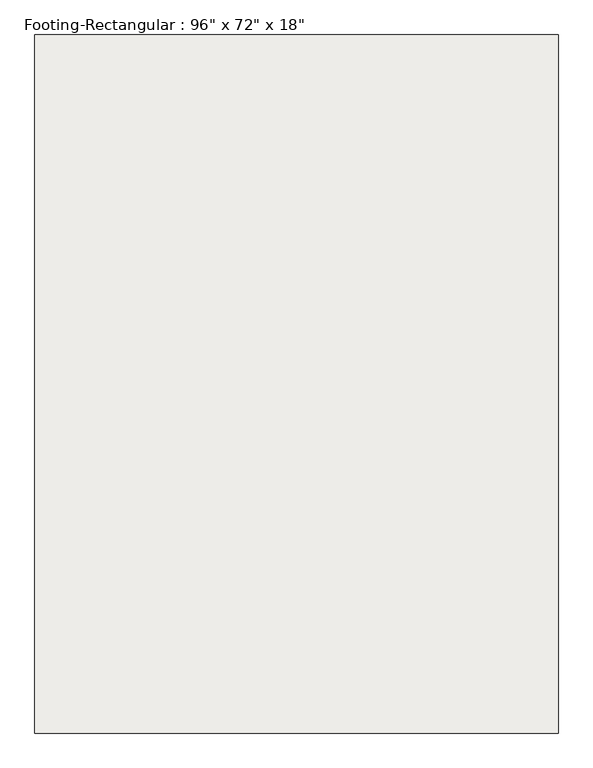
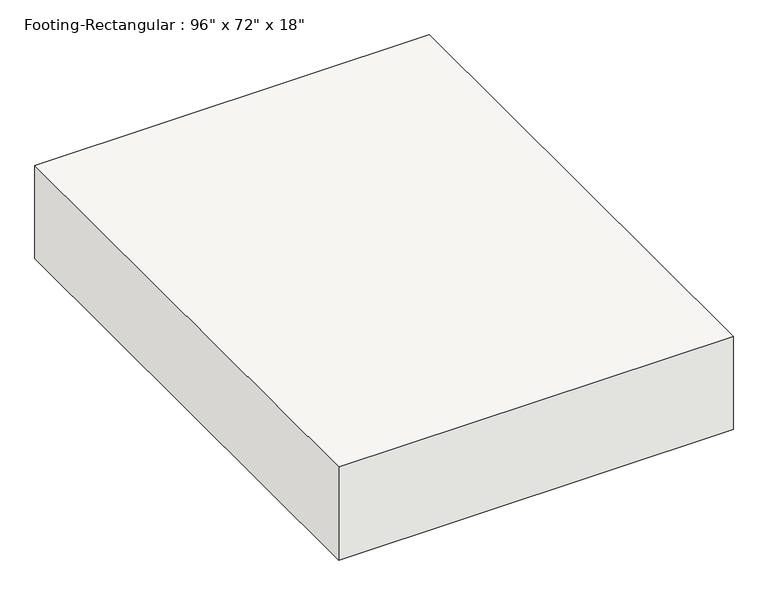
"""IFC4 building model written with IfcOpenShell, lengths in millimetres: slab geometry."""

from ifc_helpers import new_model, si_unit, frame, origin, place, context, project, spatial, polyline, outline, extrude, source, transform, mapped, element, save


def slab_7b69f09a(model_context):
    return source(origin(), model_context, "Body", "SweptSolid", [
        extrude(outline(polyline([(914.4, 1219.2), (914.4, -1219.2), (-914.4, -1219.2), (-914.4, 1219.2), (914.4, 1219.2)])), frame((0.0, 0.0, -457.2), z_axis=(0.0, 0.0, 1.0), x_axis=(1.0, 0.0, 0.0)), (0.0, 0.0, 1.0), 457.2),
    ])


if __name__ == "__main__":
    model = new_model("IFC4")
    model_context = context("Model", 3, world=origin())
    ifc_project = project(units=[si_unit("LENGTHUNIT", "METRE", prefix="MILLI")], contexts=[model_context])
    site = spatial("IfcSite", under=ifc_project)
    building = spatial("IfcBuilding", under=site)
    placement = place(None, origin())
    slab_shape = slab_7b69f09a(model_context)
    element("IfcSlab", 1, ObjectType="Footing-Rectangular : 96\" x 72\" x 18\"", at=placement, inside=building, context=model_context, shape_type="MappedRepresentation", body=[
        mapped(slab_shape, transform((0.0, 0.0, 0.0), x_axis=(1.0, 0.0, 0.0), y_axis=(0.0, 1.0, 0.0), z_axis=(0.0, 0.0, 1.0))),
    ])
    save(model, "model.ifc")

# Revit data of these elements
# Type "Footing-Rectangular : 96\" x 72\" x 18\""
#   Assembly Code = "A1010100"
#   Width = 1828.8 mm
#   Length = 2438.4 mm
#   Foundation Thickness = 457.2 mm
#   Structural Material [instance default] = Concrete, Cast-in-Place gray
# Element 1 (IfcSlab, "Footing-Rectangular : 96\" x 72\" x 18\"")
#   Materials on its faces: "Concrete, Cast-in-Place gray"
# Materials
#   "Concrete, Cast-in-Place gray": class "Concrete", colour RGB 192 192 192, transparency 0, Description = "Cast-in-place concrete", Cost = 0
